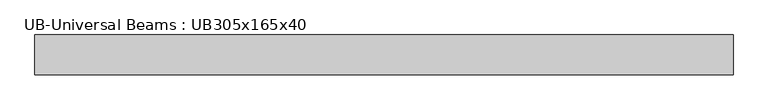
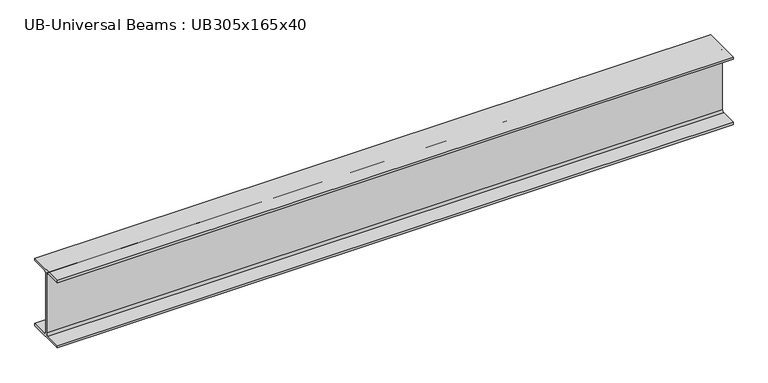
"""IFC4 building model written with IfcOpenShell, lengths in millimetres: beam geometry, UB-Universal Beams : UB305x165x40."""

from ifc_helpers import new_model, si_unit, point, frame, frame_2d, origin, place, context, project, spatial, polyline, circle_curve, trimmed, segment, composite_curve, outline, extrude, source, transform, mapped, element, save


def ub_universal_beams_ub305x165x40_f6c4464a(model_context):
    return source(origin(), model_context, "Body", "SweptSolid", [
        extrude(outline(composite_curve([segment(polyline([(82.5, -141.5), (82.5, -151.7), (-82.5, -151.7), (-82.5, -141.5), (-11.9, -141.5)]), True, "CONTINUOUS"), segment(trimmed(circle_curve(frame_2d((-11.9, -132.6)), 8.9), [point((-11.9, -141.5))], [point((-3.0, -132.6))], True, "CARTESIAN"), True, "CONTINUOUS"), segment(polyline([(-3.0, -132.6), (-3.0, 132.6)]), True, "CONTINUOUS"), segment(trimmed(circle_curve(frame_2d((-11.9, 132.6)), 8.9), [point((-3.0, 132.6))], [point((-11.9, 141.5))], True, "CARTESIAN"), True, "CONTINUOUS"), segment(polyline([(-11.9, 141.5), (-82.5, 141.5), (-82.5, 151.7), (82.5, 151.7), (82.5, 141.5), (11.9, 141.5)]), True, "CONTINUOUS"), segment(trimmed(circle_curve(frame_2d((11.9, 132.6)), 8.9), [point((11.9, 141.5))], [point((3.0, 132.6))], True, "CARTESIAN"), True, "CONTINUOUS"), segment(polyline([(3.0, 132.6), (3.0, -132.6)]), True, "CONTINUOUS"), segment(trimmed(circle_curve(frame_2d((11.9, -132.6)), 8.9), [point((3.0, -132.6))], [point((11.9, -141.5))], True, "CARTESIAN"), True, "CONTINUOUS"), segment(polyline([(11.9, -141.5), (82.5, -141.5)]), True, "CONTINUOUS")], self_intersect=False)), frame((-1387.3, 0.0, 0.0), z_axis=(1.0, 0.0, 0.0), x_axis=(0.0, 1.0, 0.0)), (0.0, 0.0, 1.0), 2874.5),
    ])


if __name__ == "__main__":
    model = new_model("IFC4")
    model_context = context("Model", 3, world=origin())
    ifc_project = project(units=[si_unit("LENGTHUNIT", "METRE", prefix="MILLI")], contexts=[model_context])
    site = spatial("IfcSite", under=ifc_project)
    building = spatial("IfcBuilding", under=site)
    placement = place(None, origin())
    ub_universal_beams_ub305x165x40_shape = ub_universal_beams_ub305x165x40_f6c4464a(model_context)
    element("IfcBeam", 1, ObjectType="UB-Universal Beams : UB305x165x40", at=placement, inside=building, context=model_context, shape_type="MappedRepresentation", body=[
        mapped(ub_universal_beams_ub305x165x40_shape, transform((0.0, 0.0, 0.0), x_axis=(1.0, 0.0, 0.0), y_axis=(0.0, 1.0, 0.0), z_axis=(0.0, 0.0, 1.0))),
    ])
    save(model, "model.ifc")

# Revit data of these elements
# Type "UB-Universal Beams : UB305x165x40"
#   Section Name Key = "UB305X165X40"
#   Width = 16.5 cm
#   Web Thickness = 0.6 cm
#   Web Fillet = 0.89 cm
#   Warping Constant = 164000.0 cm⁶
#   Torsional Moment of Inertia = 14.70 cm⁴
#   Section Area = 51.3 cm²
#   Plastic Modulus weak axis = 142.0 cm³
#   Plastic Modulus strong axis = 623.0 cm³
#   Nominal Weight = 40.2999 kgf/m
#   Moment of Inertia weak axis = 764.00 cm⁴
#   Moment of Inertia strong axis = 8503.00 cm⁴
#   Height = 30.34 cm
#   Flange Thickness = 1.02 cm
#   Elastic Modulus weak axis = 92.6 cm³
#   Elastic Modulus strong axis = 560.0 cm³
#   Centroid Vertical = 15.17 cm
#   Centroid Horizontal = 8.25 cm
#   Bolt Spacing = 9.0 cm
#   Length [instance default] = 1.5 m
#   Structural Material [instance default] = Metal - Steel 43-275
#   Type Comments = ""
#   Assembly Code = ""
# Element 1 (IfcBeam, "UB-Universal Beams : UB305x165x40")
#   Materials on its faces: "Metal - Steel 43-275"
# Materials
#   "Metal - Steel 43-275": class "Metal", colour RGB 247 247 247, transparency 0, Cost = 0
